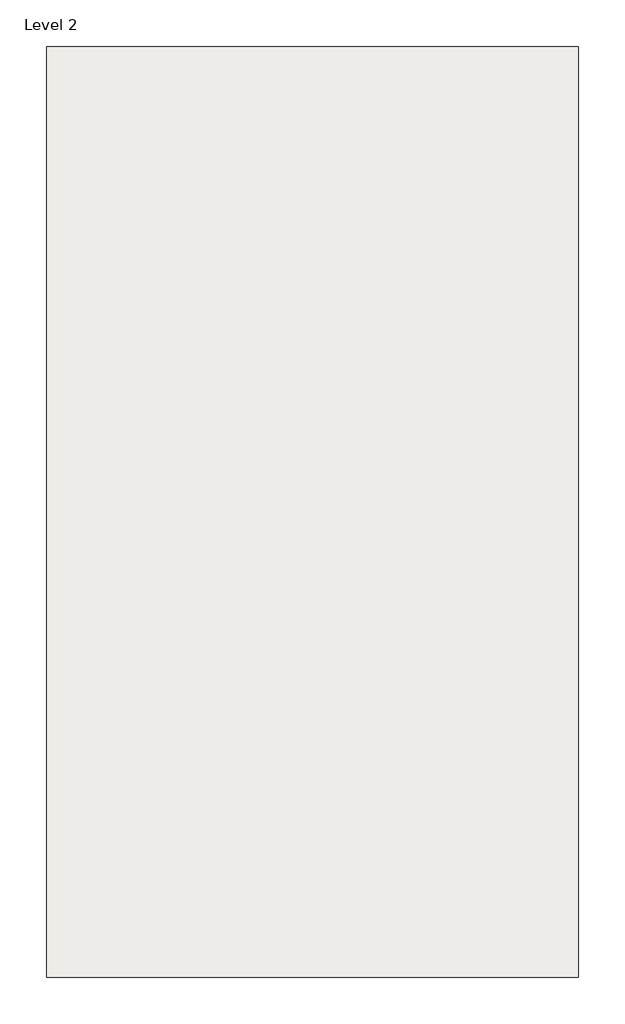
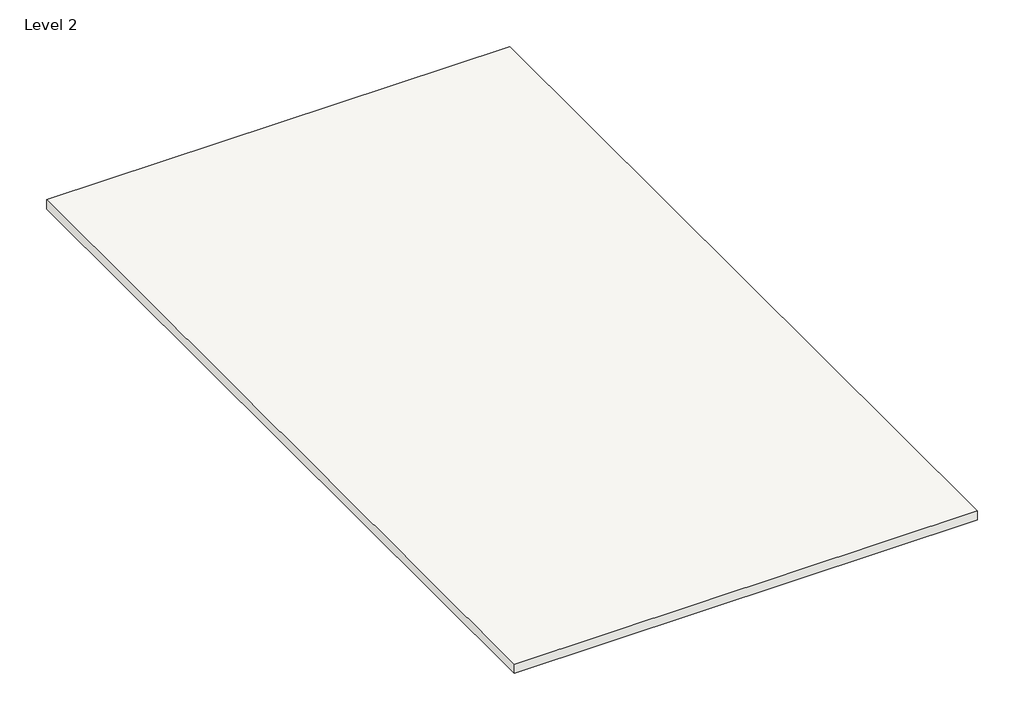
# One storey, incomplete: 1 roof.
"""IFC4 building model written with IfcOpenShell, lengths in millimetres."""

from ifc_helpers import new_model, si_unit, frame, origin, place, context, project, spatial, polyline, outline, extrude, element, save

model = new_model("IFC4")

# Units and contexts
model_context = context("Model", 3, world=origin())
ifc_project = project(units=[si_unit("LENGTHUNIT", "METRE", prefix="MILLI")], contexts=[model_context])

# Site, building, storey
site = spatial("IfcSite", under=ifc_project)
building = spatial("IfcBuilding", under=site)
storey = spatial("IfcBuildingStorey", under=building, Name="Level 2", Elevation=3048.0)

# Roof
placement = place(None, origin())
element("IfcRoof", 1, ObjectType="Generic - 12\"", at=placement, inside=storey, context=model_context, shape_type="SweptSolid", body=[
    extrude(outline(polyline([(-4881.0915084, 7034.2435985), (2370.6084916, 7034.2435985), (2370.6084916, -5653.0564015), (-4881.0915084, -5653.0564015), (-4881.0915084, 7034.2435985)])), frame((0.0, 0.0, 3048.0), z_axis=(0.0, 0.0, 1.0), x_axis=(1.0, 0.0, 0.0)), (0.0, 0.0, 1.0), 152.4),
])

save(model, "model.ifc")

# Revit data of these elements
# Type "Generic - 12\""
#   Assembly Code = "B1020"
#   Layers, outside or top first: 0' - 6" no material (function 1)
# Element 1 (IfcRoof, "Generic - 12\"")
#   built-in parameter 1001705 = 10.5 (stored number, unit not read)
#   built-in parameter 1001710 = 33615
#   Phase Created = New Construction
#   Materials on its faces: "Default Roof"
# Materials
#   "Default Roof": colour RGB 88 101 114, transparency 0, Cost = 0
